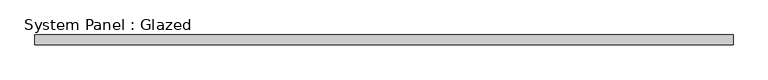
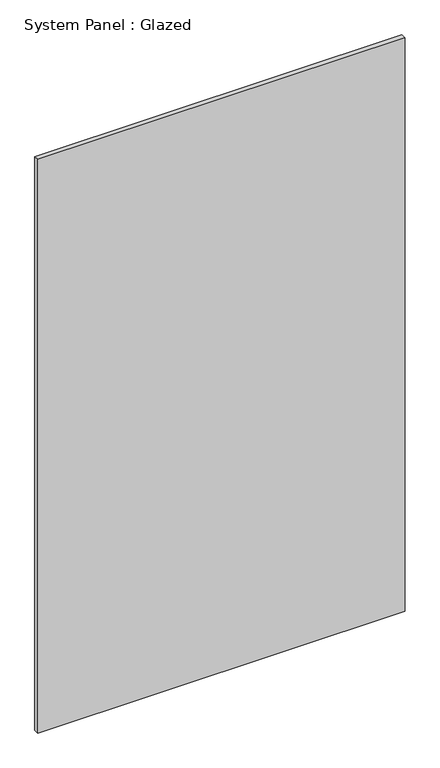
"""IFC4 building model written with IfcOpenShell, lengths in millimetres: plate geometry, System Panel : Glazed."""

from ifc_helpers import new_model, si_unit, origin, origin_with_axes, place, context, project, spatial, polyline, outline, extrude, source, transform, mapped, element, save


def system_panel_glazed_b6b14daa(model_context):
    return source(origin(), model_context, "Body", "SweptSolid", [
        extrude(outline(polyline([(908.466, 24.5), (-908.466, 24.5), (-908.466, 49.5), (908.466, 49.5), (908.466, 24.5)])), origin_with_axes(), (0.0, 0.0, 1.0), 3000.0),
    ])


if __name__ == "__main__":
    model = new_model("IFC4")
    model_context = context("Model", 3, world=origin())
    ifc_project = project(units=[si_unit("LENGTHUNIT", "METRE", prefix="MILLI")], contexts=[model_context])
    site = spatial("IfcSite", under=ifc_project)
    building = spatial("IfcBuilding", under=site)
    placement = place(None, origin())
    system_panel_glazed_shape = system_panel_glazed_b6b14daa(model_context)
    element("IfcPlate", 1, ObjectType="System Panel : Glazed", at=placement, inside=building, context=model_context, shape_type="MappedRepresentation", body=[
        mapped(system_panel_glazed_shape, transform((0.0, 0.0, 0.0), x_axis=(1.0, 0.0, 0.0), y_axis=(0.0, 1.0, 0.0), z_axis=(0.0, 0.0, 1.0))),
    ])
    save(model, "model.ifc")

# Revit data of these elements
# Type "System Panel : Glazed"
#   Keynote = "H11"
#   Construction Type Id = "GSP4R"
#   Analytic Construction = "1/8 in Pilkington single glazing"
#   Visual Light Transmittance = 0.9
#   Solar Heat Gain Coefficient = 0.86
#   Heat Transfer Coefficient (U) = 6.7069 W/(m²·K)
#   Define Thermal Properties by = 1
# Element 1 (IfcPlate, "System Panel : Glazed")
#   Materials on its faces: "Glass"
# Materials
#   "Glass": class "Glass", colour RGB 0 128 192, transparency 0.9, Description = "Soda Lime Glass", Cost = 0
